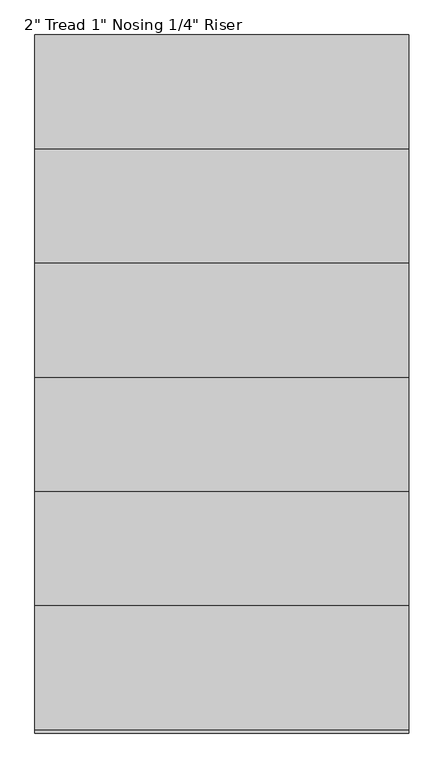
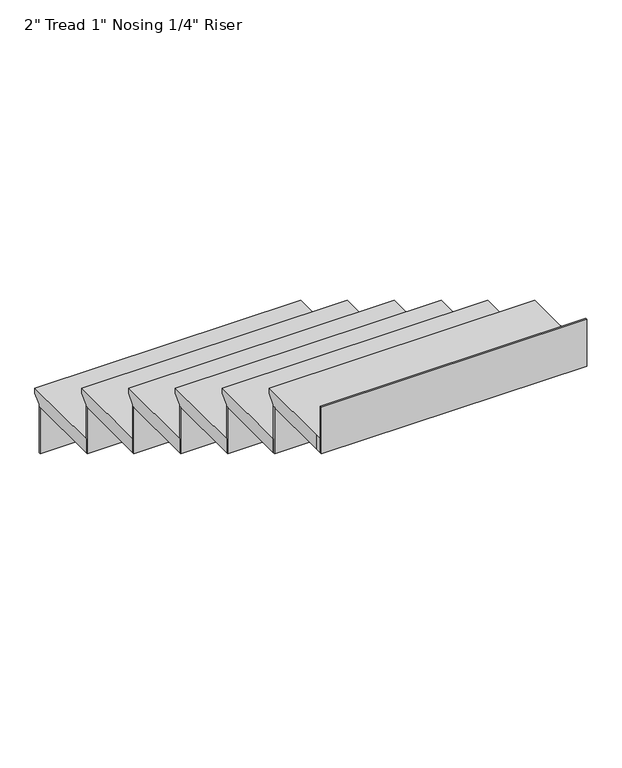
"""IFC4 building model written with IfcOpenShell, lengths in millimetres: stair flight geometry."""

from ifc_helpers import new_model, si_unit, origin, place, context, project, spatial, faceted_brep, source, transform, mapped, element, save


def stair_flight_52aa9efe(model_context):
    return source(origin(), model_context, "Body", "Brep", [
        faceted_brep([(-11268.1522729, -356.3993654, 4349.75), (-11268.1522729, -356.3993654, 4368.8), (-10353.7522729, -356.3993654, 4368.8), (-10353.7522729, -356.3993654, 4349.75), (-11268.1522729, -381.7993654, 4324.35), (-10353.7522729, -381.7993654, 4324.35), (-11268.1522729, -661.1993654, 4368.8), (-10353.7522729, -661.1993654, 4368.8), (-10353.7522729, -381.7993654, 4318.0), (-10353.7522729, -661.1993654, 4318.0), (-11268.1522729, -661.1993654, 4318.0), (-11268.1522729, -381.7993654, 4318.0)], [[[0, 1, 2, 3]], [[4, 0, 3, 5]], [[2, 1, 6, 7]], [[8, 9, 10, 11]], [[2, 7, 9, 8, 5, 3]], [[8, 11, 4, 5]], [[6, 1, 0, 4, 11, 10]], [[7, 6, 10, 9]]]),
        faceted_brep([(-11268.1522729, -381.7993654, 4318.0), (-11268.1522729, -381.7993654, 4148.6666667), (-11268.1522729, -388.1493654, 4148.6666667), (-11268.1522729, -388.1493654, 4318.0), (-10353.7522729, -381.7993654, 4318.0), (-10353.7522729, -388.1493654, 4318.0), (-10353.7522729, -388.1493654, 4148.6666667), (-10353.7522729, -381.7993654, 4148.6666667)], [[[0, 1, 2, 3]], [[4, 5, 6, 7]], [[1, 0, 4, 7]], [[2, 1, 7, 6]], [[3, 2, 6, 5]], [[0, 3, 5, 4]]]),
        faceted_brep([(-11268.1522729, -661.1993654, 4487.3333333), (-11268.1522729, -661.1993654, 4318.0), (-11268.1522729, -667.5493654, 4318.0), (-11268.1522729, -667.5493654, 4487.3333333), (-10353.7522729, -661.1993654, 4487.3333333), (-10353.7522729, -667.5493654, 4487.3333333), (-10353.7522729, -667.5493654, 4318.0), (-10353.7522729, -661.1993654, 4318.0)], [[[0, 1, 2, 3]], [[4, 5, 6, 7]], [[1, 0, 4, 7]], [[2, 1, 7, 6]], [[3, 2, 6, 5]], [[0, 3, 5, 4]]]),
        faceted_brep([(-10353.7522729, -635.7993654, 4538.1333333), (-11268.1522729, -635.7993654, 4538.1333333), (-11268.1522729, -940.5993654, 4538.1333333), (-10353.7522729, -940.5993654, 4538.1333333), (-10353.7522729, -661.1993654, 4487.3333333), (-10353.7522729, -940.5993654, 4487.3333333), (-11268.1522729, -940.5993654, 4487.3333333), (-11268.1522729, -661.1993654, 4487.3333333), (-10353.7522729, -661.1993654, 4493.6833333), (-10353.7522729, -635.7993654, 4519.0833333), (-11268.1522729, -661.1993654, 4493.6833333), (-11268.1522729, -635.7993654, 4519.0833333)], [[[0, 1, 2, 3]], [[4, 5, 6, 7]], [[0, 3, 5, 4, 8, 9]], [[4, 7, 10, 8]], [[2, 1, 11, 10, 7, 6]], [[3, 2, 6, 5]], [[11, 1, 0, 9]], [[10, 11, 9, 8]]]),
        faceted_brep([(-11268.1522729, -940.5993654, 4656.6666667), (-11268.1522729, -940.5993654, 4487.3333333), (-11268.1522729, -946.9493654, 4487.3333333), (-11268.1522729, -946.9493654, 4656.6666667), (-10353.7522729, -940.5993654, 4656.6666667), (-10353.7522729, -946.9493654, 4656.6666667), (-10353.7522729, -946.9493654, 4487.3333333), (-10353.7522729, -940.5993654, 4487.3333333)], [[[0, 1, 2, 3]], [[4, 5, 6, 7]], [[1, 0, 4, 7]], [[2, 1, 7, 6]], [[3, 2, 6, 5]], [[0, 3, 5, 4]]]),
        faceted_brep([(-10353.7522729, -915.1993654, 4707.4666667), (-11268.1522729, -915.1993654, 4707.4666667), (-11268.1522729, -1219.9993654, 4707.4666667), (-10353.7522729, -1219.9993654, 4707.4666667), (-10353.7522729, -940.5993654, 4656.6666667), (-10353.7522729, -1219.9993654, 4656.6666667), (-11268.1522729, -1219.9993654, 4656.6666667), (-11268.1522729, -940.5993654, 4656.6666667), (-10353.7522729, -940.5993654, 4663.0166667), (-10353.7522729, -915.1993654, 4688.4166667), (-11268.1522729, -940.5993654, 4663.0166667), (-11268.1522729, -915.1993654, 4688.4166667)], [[[0, 1, 2, 3]], [[4, 5, 6, 7]], [[0, 3, 5, 4, 8, 9]], [[4, 7, 10, 8]], [[2, 1, 11, 10, 7, 6]], [[3, 2, 6, 5]], [[11, 1, 0, 9]], [[10, 11, 9, 8]]]),
        faceted_brep([(-11268.1522729, -1219.9993654, 4826.0), (-11268.1522729, -1219.9993654, 4656.6666667), (-11268.1522729, -1226.3493654, 4656.6666667), (-11268.1522729, -1226.3493654, 4826.0), (-10353.7522729, -1219.9993654, 4826.0), (-10353.7522729, -1226.3493654, 4826.0), (-10353.7522729, -1226.3493654, 4656.6666667), (-10353.7522729, -1219.9993654, 4656.6666667)], [[[0, 1, 2, 3]], [[4, 5, 6, 7]], [[1, 0, 4, 7]], [[2, 1, 7, 6]], [[3, 2, 6, 5]], [[0, 3, 5, 4]]]),
        faceted_brep([(-10353.7522729, -1194.5993654, 4876.8), (-11268.1522729, -1194.5993654, 4876.8), (-11268.1522729, -1499.3993654, 4876.8), (-10353.7522729, -1499.3993654, 4876.8), (-10353.7522729, -1219.9993654, 4826.0), (-10353.7522729, -1499.3993654, 4826.0), (-11268.1522729, -1499.3993654, 4826.0), (-11268.1522729, -1219.9993654, 4826.0), (-10353.7522729, -1219.9993654, 4832.35), (-10353.7522729, -1194.5993654, 4857.75), (-11268.1522729, -1219.9993654, 4832.35), (-11268.1522729, -1194.5993654, 4857.75)], [[[0, 1, 2, 3]], [[4, 5, 6, 7]], [[0, 3, 5, 4, 8, 9]], [[4, 7, 10, 8]], [[2, 1, 11, 10, 7, 6]], [[3, 2, 6, 5]], [[11, 1, 0, 9]], [[10, 11, 9, 8]]]),
        faceted_brep([(-11268.1522729, -1499.3993654, 4995.3333333), (-11268.1522729, -1499.3993654, 4826.0), (-11268.1522729, -1505.7493654, 4826.0), (-11268.1522729, -1505.7493654, 4995.3333333), (-10353.7522729, -1499.3993654, 4995.3333333), (-10353.7522729, -1505.7493654, 4995.3333333), (-10353.7522729, -1505.7493654, 4826.0), (-10353.7522729, -1499.3993654, 4826.0)], [[[0, 1, 2, 3]], [[4, 5, 6, 7]], [[1, 0, 4, 7]], [[2, 1, 7, 6]], [[3, 2, 6, 5]], [[0, 3, 5, 4]]]),
        faceted_brep([(-10353.7522729, -1473.9993654, 5046.1333333), (-11268.1522729, -1473.9993654, 5046.1333333), (-11268.1522729, -1778.7993654, 5046.1333333), (-10353.7522729, -1778.7993654, 5046.1333333), (-10353.7522729, -1499.3993654, 4995.3333333), (-10353.7522729, -1778.7993654, 4995.3333333), (-11268.1522729, -1778.7993654, 4995.3333333), (-11268.1522729, -1499.3993654, 4995.3333333), (-10353.7522729, -1499.3993654, 5001.6833333), (-10353.7522729, -1473.9993654, 5027.0833333), (-11268.1522729, -1499.3993654, 5001.6833333), (-11268.1522729, -1473.9993654, 5027.0833333)], [[[0, 1, 2, 3]], [[4, 5, 6, 7]], [[0, 3, 5, 4, 8, 9]], [[4, 7, 10, 8]], [[2, 1, 11, 10, 7, 6]], [[3, 2, 6, 5]], [[11, 1, 0, 9]], [[10, 11, 9, 8]]]),
        faceted_brep([(-11268.1522729, -2058.1993654, 5334.0), (-11268.1522729, -2058.1993654, 5164.6666667), (-11268.1522729, -2064.5493654, 5164.6666667), (-11268.1522729, -2064.5493654, 5334.0), (-10353.7522729, -2058.1993654, 5334.0), (-10353.7522729, -2064.5493654, 5334.0), (-10353.7522729, -2064.5493654, 5164.6666667), (-10353.7522729, -2058.1993654, 5164.6666667)], [[[0, 1, 2, 3]], [[4, 5, 6, 7]], [[1, 0, 4, 7]], [[2, 1, 7, 6]], [[3, 2, 6, 5]], [[0, 3, 5, 4]]]),
        faceted_brep([(-11268.1522729, -1778.7993654, 5164.6666667), (-11268.1522729, -1778.7993654, 4995.3333333), (-11268.1522729, -1785.1493654, 4995.3333333), (-11268.1522729, -1785.1493654, 5164.6666667), (-10353.7522729, -1778.7993654, 5164.6666667), (-10353.7522729, -1785.1493654, 5164.6666667), (-10353.7522729, -1785.1493654, 4995.3333333), (-10353.7522729, -1778.7993654, 4995.3333333)], [[[0, 1, 2, 3]], [[4, 5, 6, 7]], [[1, 0, 4, 7]], [[2, 1, 7, 6]], [[3, 2, 6, 5]], [[0, 3, 5, 4]]]),
        faceted_brep([(-10353.7522729, -1753.3993654, 5215.4666667), (-11268.1522729, -1753.3993654, 5215.4666667), (-11268.1522729, -2032.7993654, 5215.4666667), (-11268.1522729, -2058.1993654, 5215.4666667), (-10353.7522729, -2058.1993654, 5215.4666667), (-10353.7522729, -1778.7993654, 5164.6666667), (-10353.7522729, -2058.1993654, 5164.6666667), (-11268.1522729, -2058.1993654, 5164.6666667), (-11268.1522729, -2032.7993654, 5164.6666667), (-11268.1522729, -1778.7993654, 5164.6666667), (-10353.7522729, -1778.7993654, 5171.0166667), (-10353.7522729, -1753.3993654, 5196.4166667), (-11268.1522729, -1778.7993654, 5171.0166667), (-11268.1522729, -1753.3993654, 5196.4166667)], [[[0, 1, 2, 3, 4]], [[5, 6, 7, 8, 9]], [[0, 4, 6, 5, 10, 11]], [[5, 9, 12, 10]], [[2, 1, 13, 12, 9, 8]], [[3, 2, 8, 7]], [[4, 3, 7, 6]], [[13, 1, 0, 11]], [[12, 13, 11, 10]]]),
    ])


if __name__ == "__main__":
    model = new_model("IFC4")
    model_context = context("Model", 3, world=origin())
    ifc_project = project(units=[si_unit("LENGTHUNIT", "METRE", prefix="MILLI")], contexts=[model_context])
    site = spatial("IfcSite", under=ifc_project)
    building = spatial("IfcBuilding", under=site)
    placement = place(None, origin())
    stair_flight_shape = stair_flight_52aa9efe(model_context)
    element("IfcStairFlight", 1, ObjectType="2\" Tread 1\" Nosing 1/4\" Riser", at=placement, inside=building, context=model_context, shape_type="MappedRepresentation", body=[
        mapped(stair_flight_shape, transform((0.0, 0.0, 0.0), x_axis=(1.0, 0.0, 0.0), y_axis=(0.0, 1.0, 0.0), z_axis=(0.0, 0.0, 1.0))),
    ])
    save(model, "model.ifc")
